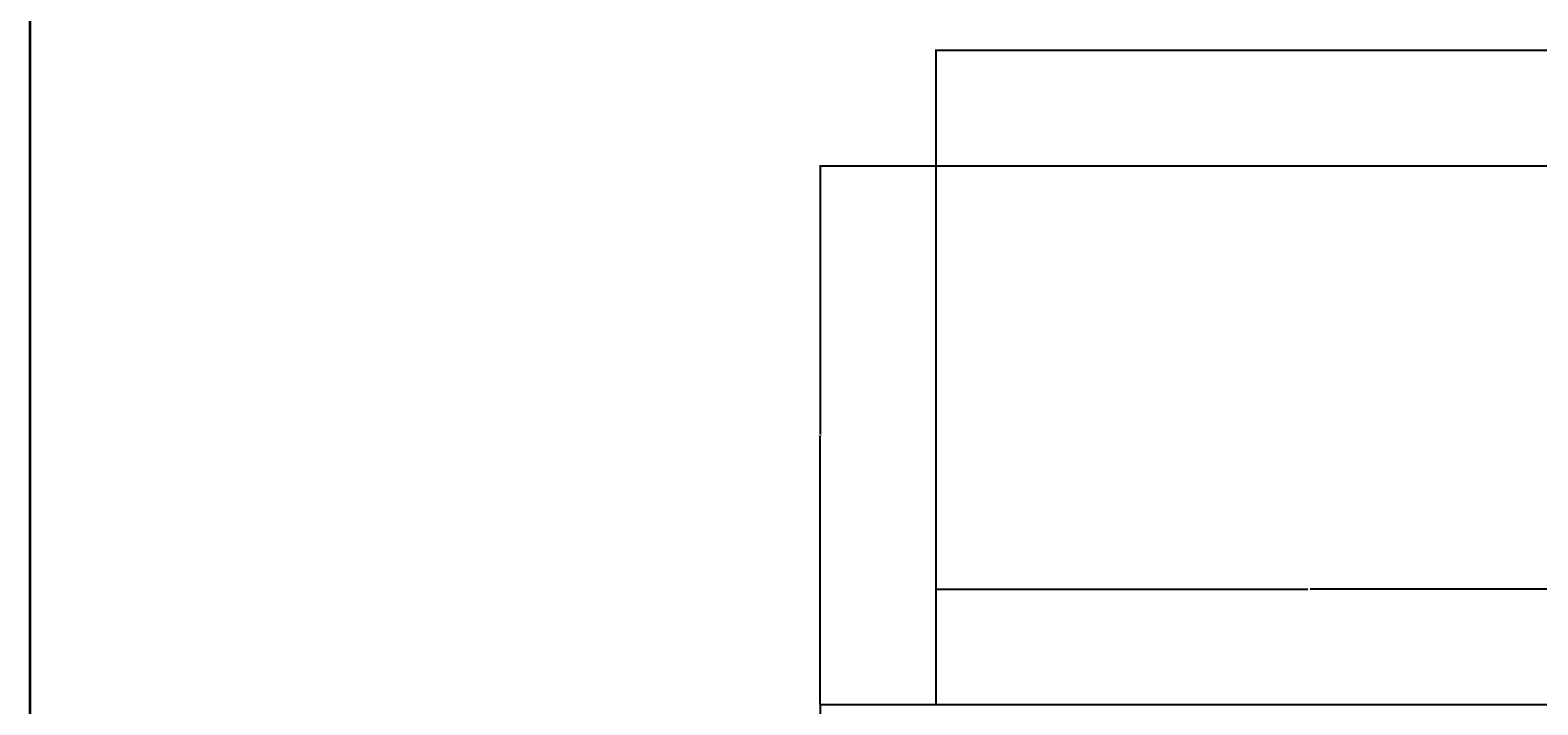
# Model space of a CAD drawing. Units: inches. Extents: x 2067 to 3463, y 1605 to 2723.
# Tile 3 of 10: x 2067 to 2403, y 2038 to 2189. Entities that reach past the tile are written whole.
import ezdxf

# ---------------------------------------------------------------- set-up
doc = ezdxf.new("R2010")
doc.units = ezdxf.units.IN
doc.layers.add('A-ANNO-DIMS', color=2, linetype='Continuous', lineweight=18)
doc.layers.add('A-ANNO-TTLB', color=7, linetype='Continuous', lineweight=35)
doc.styles.get("Standard").update_dxf_attribs({"font": 'arial.ttf'})
doc.dimstyles.get("Standard").update_dxf_attribs({"dimtxt": 0.18, "dimasz": 0.18, "dimexe": 0.18, "dimexo": 0.0625, "dimgap": 0.09, "dimtad": 0, "dimtih": 1, "dimtoh": 1, "dimdec": 4, "dimzin": 0, "dimdsep": 46, "dimtxsty": 'Standard', "dimcen": 0.09, "dimadec": 0, "dimazin": 0, "dimtfac": 1, "dimtdec": 4, "dimtofl": 0, "dimtmove": 0, "dimatfit": 3, "dimfxl": 1, "dimtolj": 1, "dimtzin": 0, "dimarcsym": 0})

# ---------------------------------------------------------------- blocks, each defined once
blk = doc.blocks.new('*D28')
at = {"layer": 'A-ANNO-DIMS', "color": 0, "lineweight": -2, "transparency": 16777216}
for p, q in [((2268.95, 2038.28), (2268.95, 2184.21)), ((2269.13, 2184.03), (2487.3, 2184.03)), ((2706.27, 2184.03), (2488.1, 2184.03)), ((2706.45, 2158.29), (2706.45, 2184.21))]:
    blk.add_line(p, q, dxfattribs=at)
at = {"layer": 'A-ANNO-DIMS', "color": 0, "transparency": 16777216}
for points in [[(2269.13, 2184.06), (2269.13, 2184), (2268.95, 2184.03)], [(2706.27, 2184.06), (2706.27, 2184), (2706.45, 2184.03)]]:
    blk.add_solid(points, dxfattribs=at)
at = {"layer": 'Defpoints', "color": 0, "transparency": 16777216}
for p in [(2706.45, 2184.03), (2706.45, 2158.23), (2268.95, 2038.22)]:
    blk.add_point(p, dxfattribs=at)
at = {"layer": 'A-ANNO-DIMS', "color": 0, "transparency": 16777216, "insert": (2487.7, 2184.03), "char_height": 0.18, "attachment_point": 5}
blk.add_mtext('\\A1;437.5', dxfattribs=at)
blk = doc.blocks.new('*D30')
at = {"layer": 'A-ANNO-DIMS', "color": 0, "lineweight": -2, "transparency": 16777216}
for p, q in [((2268.95, 2038.28), (2268.95, 2064.2)), ((2269.13, 2064.02), (2351.67, 2064.02)), ((2434.77, 2064.02), (2352.23, 2064.02)), ((2434.95, 2038.28), (2434.95, 2064.2))]:
    blk.add_line(p, q, dxfattribs=at)
at = {"layer": 'A-ANNO-DIMS', "color": 0, "transparency": 16777216}
for points in [[(2269.13, 2064.05), (2269.13, 2063.99), (2268.95, 2064.02)], [(2434.77, 2064.05), (2434.77, 2063.99), (2434.95, 2064.02)]]:
    blk.add_solid(points, dxfattribs=at)
at = {"layer": 'Defpoints', "color": 0, "transparency": 16777216}
for p in [(2434.95, 2064.02), (2268.95, 2038.22), (2434.95, 2038.22)]:
    blk.add_point(p, dxfattribs=at)
at = {"layer": 'A-ANNO-DIMS', "color": 0, "transparency": 16777216, "insert": (2351.95, 2064.02), "char_height": 0.18, "attachment_point": 5}
blk.add_mtext('\\A1;166', dxfattribs=at)
blk = doc.blocks.new('*D31')
at = {"layer": 'A-ANNO-DIMS', "color": 0, "lineweight": -2, "transparency": 16777216}
for p, q in [((2434.89, 2158.23), (2242.97, 2158.23)), ((2243.15, 2158.05), (2243.15, 2098.41)), ((2243.15, 2038.4), (2243.15, 2098.04)), ((2434.89, 2038.22), (2242.97, 2038.22))]:
    blk.add_line(p, q, dxfattribs=at)
at = {"layer": 'A-ANNO-DIMS', "color": 0, "transparency": 16777216}
for points in [[(2243.12, 2158.05), (2243.18, 2158.05), (2243.15, 2158.23)], [(2243.12, 2038.4), (2243.18, 2038.4), (2243.15, 2038.22)]]:
    blk.add_solid(points, dxfattribs=at)
at = {"layer": 'Defpoints', "color": 0, "transparency": 16777216}
for p in [(2243.15, 2158.23), (2434.95, 2158.23), (2434.95, 2038.22)]:
    blk.add_point(p, dxfattribs=at)
at = {"layer": 'A-ANNO-DIMS', "color": 0, "transparency": 16777216, "insert": (2243.15, 2098.22), "char_height": 0.18, "attachment_point": 5}
blk.add_mtext('\\A1;120.01', dxfattribs=at)
blk = doc.blocks.new('*D32')
at = {"layer": 'A-ANNO-DIMS', "color": 0, "lineweight": -2, "transparency": 16777216}
for p, q in [((2268.89, 2038.22), (2242.97, 2038.22)), ((2243.15, 2038.04), (2243.15, 2022.47)), ((2243.15, 2006.54), (2243.15, 2022.11)), ((2268.89, 2006.36), (2242.97, 2006.36))]:
    blk.add_line(p, q, dxfattribs=at)
at = {"layer": 'A-ANNO-DIMS', "color": 0, "transparency": 16777216}
for points in [[(2243.12, 2038.04), (2243.18, 2038.04), (2243.15, 2038.22)], [(2243.12, 2006.54), (2243.18, 2006.54), (2243.15, 2006.36)]]:
    blk.add_solid(points, dxfattribs=at)
at = {"layer": 'Defpoints', "color": 0, "transparency": 16777216}
for p in [(2243.15, 2038.22), (2268.95, 2038.22), (2268.95, 2006.36)]:
    blk.add_point(p, dxfattribs=at)
at = {"layer": 'A-ANNO-DIMS', "color": 0, "transparency": 16777216, "insert": (2243.15, 2022.29), "char_height": 0.18, "attachment_point": 5}
blk.add_mtext('\\A1;31.86', dxfattribs=at)

msp = doc.modelspace()

# ---------------------------------------------------------------- linework, layer by layer
at = {"layer": 'A-ANNO-TTLB'}
msp.add_lwpolyline([(2067.2624, 2722.6321), (3463.3053, 2722.6321), (3463.3053, 1605.3918), (2067.2624, 1605.3918)], close=True, dxfattribs=at)

# ---------------------------------------------------------------- dimensions: what is measured, and where the dimension line sits
at = {"layer": 'A-ANNO-DIMS'}
for base, p2, override, picture, middle in [((2706.4477, 2184.0309), (2706.4477, 2158.2309), {"dimdec": 1, "dimlfac": 1, "dimrnd": 0, "dimzin": 0, "dimdsep": 46, "dimlunit": 2}, '*D28', (2487.6977, 2184.0309)), ((2434.9477, 2064.0171), (2434.9477, 2038.2171), {"dimdec": 0, "dimlfac": 1, "dimrnd": 0, "dimzin": 0, "dimdsep": 46, "dimlunit": 2}, '*D30', (2351.9477, 2064.0171))]:
    dim = msp.add_linear_dim(base=base, p1=(2268.9477, 2038.2171), p2=p2, dimstyle='Standard', override=override, dxfattribs=at)
    dim.commit()
    dim.dimension.update_dxf_attribs({"geometry": picture, "text_midpoint": middle})
for base, p1, p2, picture, middle in [((2243.1477, 2158.2309), (2434.9477, 2038.2171), (2434.9477, 2158.2309), '*D31', (2243.1477, 2098.224)), ((2243.1477, 2038.2171), (2268.9477, 2006.3591), (2268.9477, 2038.2171), '*D32', (2243.1477, 2022.2881))]:
    dim = msp.add_linear_dim(base=base, p1=p1, p2=p2, angle=90, dimstyle='Standard', override={"dimdec": 2, "dimlfac": 1, "dimrnd": 0, "dimzin": 0, "dimdsep": 46, "dimlunit": 2}, dxfattribs=at)
    dim.commit()
    dim.dimension.update_dxf_attribs({"geometry": picture, "text_midpoint": middle})

doc.saveas('drawing.dxf')
